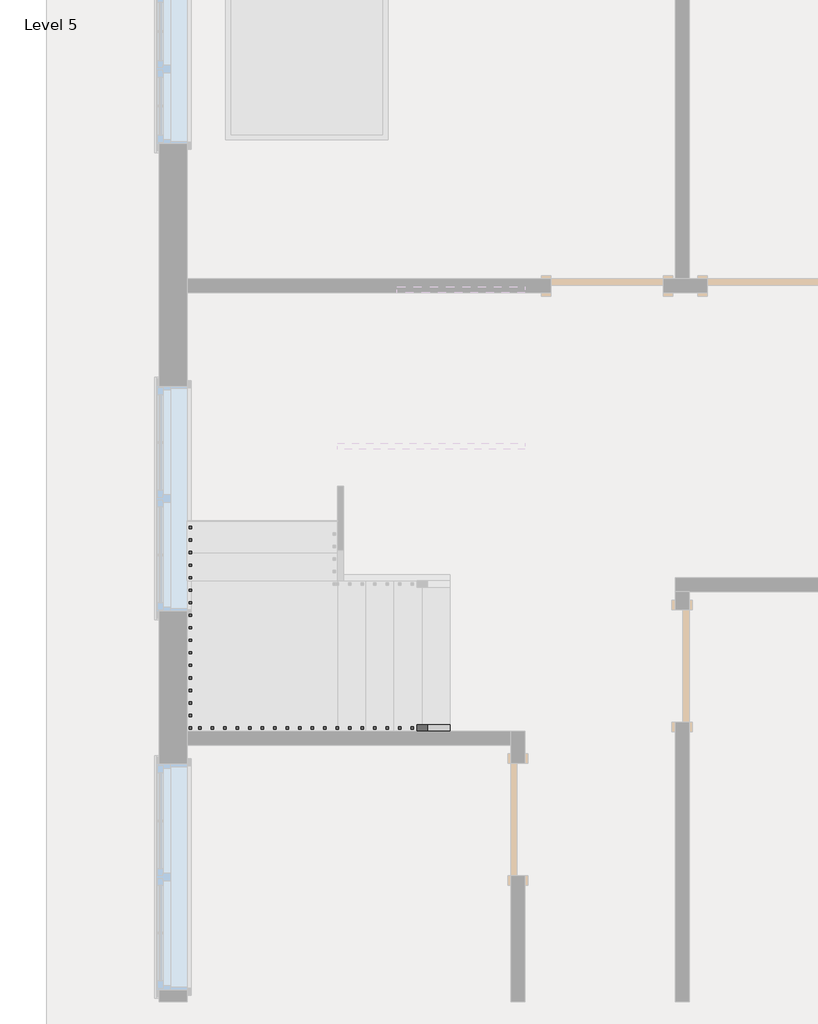
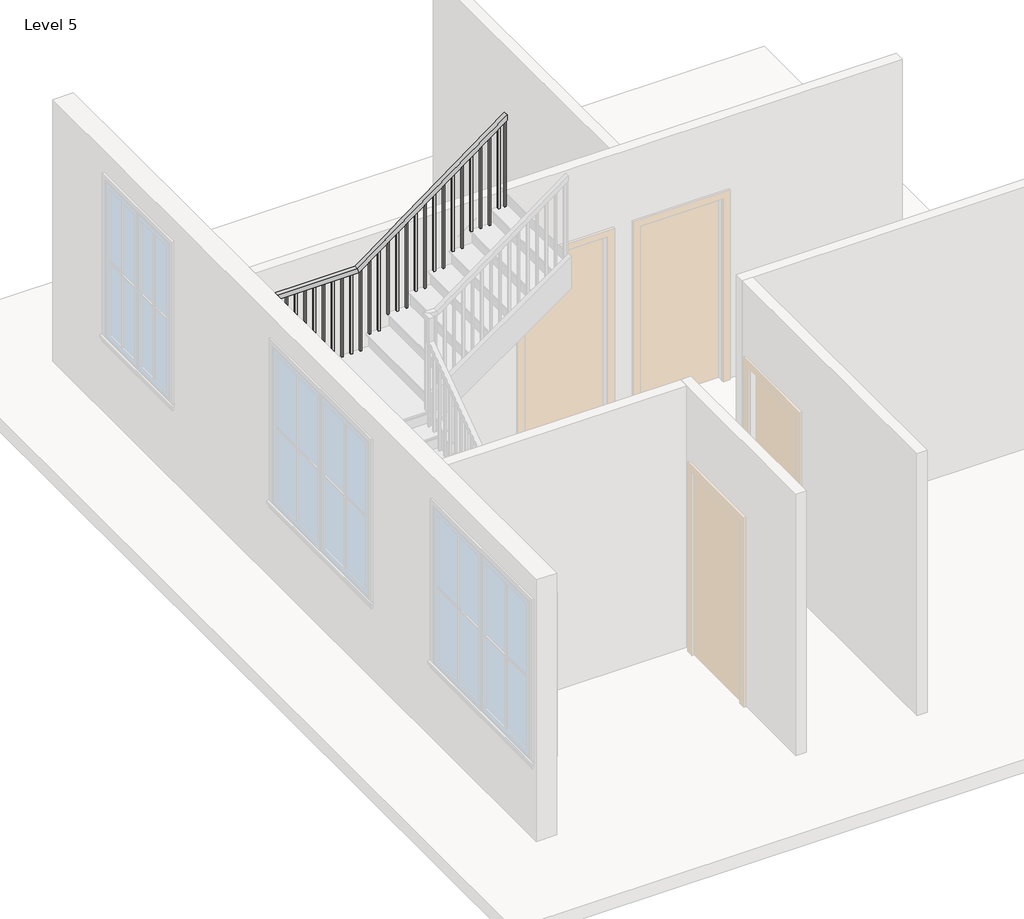
# One storey, part 2 of 3: 1 railing.
"""IFC4 building model written with IfcOpenShell, lengths in millimetres."""

from ifc_helpers import new_model, si_unit, frame, origin, place, context, project, spatial, polyline, outline, extrude, faceted_brep, element, save

model = new_model("IFC4")

# Units and contexts
model_context = context("Model", 3, world=origin())
ifc_project = project(units=[si_unit("LENGTHUNIT", "METRE", prefix="MILLI")], contexts=[model_context])

# Site, building, storey
site = spatial("IfcSite", under=ifc_project)
building = spatial("IfcBuilding", under=site)
storey = spatial("IfcBuildingStorey", under=building, Name="Level 5", Elevation=12649.2)

# Railing
placement = place(None, origin())
element("IfcRailing", 1, ObjectType="Handrail - Rectangular", at=placement, inside=storey, context=model_context, shape_type="SolidModel", body=[
    faceted_brep([(-2683.1105391, -2741.0373761, 13724.0210526), (-2683.1105391, -2741.0373761, 13661.9605986), (-2683.1105391, -2690.2373761, 13661.9605986), (-2683.1105391, -2690.2373761, 13724.0210526), (-3698.24463, -2741.0373761, 14436.3958533), (-3714.290777, -2741.0373761, 14385.5958533), (-3714.290777, -2690.2373761, 14385.5958533), (-3698.24463, -2690.2373761, 14436.3958533), (-4816.7105391, -2741.0373761, 14436.3958533), (-4816.7105391, -2741.0373761, 14385.5958533), (-4765.9105391, -2690.2373761, 14385.5958533), (-4765.9105391, -2690.2373761, 14436.3958533), (-4816.7105391, -1646.8618205, 14436.3958533), (-4816.7105391, -1630.5188912, 14385.5958533), (-4765.9105391, -1630.5188912, 14385.5958533), (-4765.9105391, -1646.8618205, 14436.3958533), (-4816.7105391, -308.3947094, 15397.0181818), (-4816.7105391, -292.0517801, 15346.2181818), (-4765.9105391, -292.0517801, 15346.2181818), (-4765.9105391, -308.3947094, 15397.0181818), (-4816.7105391, 814.9626239, 15397.0181818), (-4816.7105391, 814.9626239, 15346.2181818), (-4765.9105391, 764.1626239, 15346.2181818), (-4765.9105391, 764.1626239, 15397.0181818), (-3721.871578, 814.9626239, 15397.0181818), (-3705.1770744, 814.9626239, 15346.2181818), (-3705.1770744, 764.1626239, 15346.2181818), (-3721.871578, 764.1626239, 15397.0181818), (-2073.5105391, 814.9626239, 16611.6), (-2073.5105391, 764.1626239, 16611.6), (-2073.5105391, 764.1626239, 16548.4987868), (-2073.5105391, 814.9626239, 16548.4987868)], [[[0, 1, 2, 3]], [[1, 0, 4, 5]], [[2, 1, 5, 6]], [[3, 2, 6, 7]], [[0, 3, 7, 4]], [[5, 4, 8, 9]], [[6, 5, 9, 10]], [[7, 6, 10, 11]], [[4, 7, 11, 8]], [[9, 8, 12, 13]], [[10, 9, 13, 14]], [[11, 10, 14, 15]], [[8, 11, 15, 12]], [[13, 12, 16, 17]], [[14, 13, 17, 18]], [[15, 14, 18, 19]], [[12, 15, 19, 16]], [[17, 16, 20, 21]], [[18, 17, 21, 22]], [[19, 18, 22, 23]], [[16, 19, 23, 20]], [[21, 20, 24, 25]], [[22, 21, 25, 26]], [[23, 22, 26, 27]], [[20, 23, 27, 24]], [[28, 29, 30, 31]], [[25, 24, 28, 31]], [[26, 25, 31, 30]], [[27, 26, 30, 29]], [[24, 27, 29, 28]]]),
    extrude(outline(polyline([(16485.3329974, -2159.2355391), (15536.7789474, -2159.2355391), (15536.7789474, -2140.1855391), (16499.3698395, -2140.1855391), (16485.3329974, -2159.2355391)])), frame((0.0, 780.0376239, 0.0), z_axis=(0.0, 1.0, 0.0), x_axis=(0.0, 0.0, 1.0)), (0.0, 0.0, 1.0), 19.05),
    extrude(outline(polyline([(16410.4698395, -2260.8355391), (15376.3578947, -2260.8355391), (15376.3578947, -2241.7855391), (16424.5066816, -2241.7855391), (16410.4698395, -2260.8355391)])), frame((0.0, 780.0376239, 0.0), z_axis=(0.0, 1.0, 0.0), x_axis=(0.0, 0.0, 1.0)), (0.0, 0.0, 1.0), 19.05),
    extrude(outline(polyline([(16335.6066816, -2362.4355391), (15376.3578947, -2362.4355391), (15376.3578947, -2343.3855391), (16349.6435237, -2343.3855391), (16335.6066816, -2362.4355391)])), frame((0.0, 780.0376239, 0.0), z_axis=(0.0, 1.0, 0.0), x_axis=(0.0, 0.0, 1.0)), (0.0, 0.0, 1.0), 19.05),
    extrude(outline(polyline([(16260.7435237, -2464.0355391), (15376.3578947, -2464.0355391), (15376.3578947, -2444.9855391), (16274.7803658, -2444.9855391), (16260.7435237, -2464.0355391)])), frame((0.0, 780.0376239, 0.0), z_axis=(0.0, 1.0, 0.0), x_axis=(0.0, 0.0, 1.0)), (0.0, 0.0, 1.0), 19.05),
    extrude(outline(polyline([(16185.8803658, -2565.6355391), (15215.9368421, -2565.6355391), (15215.9368421, -2546.5855391), (16199.9172079, -2546.5855391), (16185.8803658, -2565.6355391)])), frame((0.0, 780.0376239, 0.0), z_axis=(0.0, 1.0, 0.0), x_axis=(0.0, 0.0, 1.0)), (0.0, 0.0, 1.0), 19.05),
    extrude(outline(polyline([(16111.0172079, -2667.2355391), (15215.9368421, -2667.2355391), (15215.9368421, -2648.1855391), (16125.05405, -2648.1855391), (16111.0172079, -2667.2355391)])), frame((0.0, 780.0376239, 0.0), z_axis=(0.0, 1.0, 0.0), x_axis=(0.0, 0.0, 1.0)), (0.0, 0.0, 1.0), 19.05),
    extrude(outline(polyline([(16036.15405, -2768.8355391), (15055.5157895, -2768.8355391), (15055.5157895, -2749.7855391), (16050.1908921, -2749.7855391), (16036.15405, -2768.8355391)])), frame((0.0, 780.0376239, 0.0), z_axis=(0.0, 1.0, 0.0), x_axis=(0.0, 0.0, 1.0)), (0.0, 0.0, 1.0), 19.05),
    extrude(outline(polyline([(15961.2908921, -2870.4355391), (15055.5157895, -2870.4355391), (15055.5157895, -2851.3855391), (15975.3277342, -2851.3855391), (15961.2908921, -2870.4355391)])), frame((0.0, 780.0376239, 0.0), z_axis=(0.0, 1.0, 0.0), x_axis=(0.0, 0.0, 1.0)), (0.0, 0.0, 1.0), 19.05),
    extrude(outline(polyline([(15886.4277342, -2972.0355391), (14895.0947368, -2972.0355391), (14895.0947368, -2952.9855391), (15900.4645763, -2952.9855391), (15886.4277342, -2972.0355391)])), frame((0.0, 780.0376239, 0.0), z_axis=(0.0, 1.0, 0.0), x_axis=(0.0, 0.0, 1.0)), (0.0, 0.0, 1.0), 19.05),
    extrude(outline(polyline([(15811.5645763, -3073.6355391), (14895.0947368, -3073.6355391), (14895.0947368, -3054.5855391), (15825.6014184, -3054.5855391), (15811.5645763, -3073.6355391)])), frame((0.0, 780.0376239, 0.0), z_axis=(0.0, 1.0, 0.0), x_axis=(0.0, 0.0, 1.0)), (0.0, 0.0, 1.0), 19.05),
    extrude(outline(polyline([(15736.7014184, -3175.2355391), (14734.6736842, -3175.2355391), (14734.6736842, -3156.1855391), (15750.7382605, -3156.1855391), (15736.7014184, -3175.2355391)])), frame((0.0, 780.0376239, 0.0), z_axis=(0.0, 1.0, 0.0), x_axis=(0.0, 0.0, 1.0)), (0.0, 0.0, 1.0), 19.05),
    extrude(outline(polyline([(15661.8382605, -3276.8355391), (14734.6736842, -3276.8355391), (14734.6736842, -3257.7855391), (15675.8751026, -3257.7855391), (15661.8382605, -3276.8355391)])), frame((0.0, 780.0376239, 0.0), z_axis=(0.0, 1.0, 0.0), x_axis=(0.0, 0.0, 1.0)), (0.0, 0.0, 1.0), 19.05),
    extrude(outline(polyline([(15586.9751026, -3378.4355391), (14734.6736842, -3378.4355391), (14734.6736842, -3359.3855391), (15601.0119447, -3359.3855391), (15586.9751026, -3378.4355391)])), frame((0.0, 780.0376239, 0.0), z_axis=(0.0, 1.0, 0.0), x_axis=(0.0, 0.0, 1.0)), (0.0, 0.0, 1.0), 19.05),
    extrude(outline(polyline([(15512.1119447, -3480.0355391), (14574.2526316, -3480.0355391), (14574.2526316, -3460.9855391), (15526.1487868, -3460.9855391), (15512.1119447, -3480.0355391)])), frame((0.0, 780.0376239, 0.0), z_axis=(0.0, 1.0, 0.0), x_axis=(0.0, 0.0, 1.0)), (0.0, 0.0, 1.0), 19.05),
    extrude(outline(polyline([(15437.2487868, -3581.6355391), (14574.2526316, -3581.6355391), (14574.2526316, -3562.5855391), (15451.2856289, -3562.5855391), (15437.2487868, -3581.6355391)])), frame((0.0, 780.0376239, 0.0), z_axis=(0.0, 1.0, 0.0), x_axis=(0.0, 0.0, 1.0)), (0.0, 0.0, 1.0), 19.05),
    extrude(outline(polyline([(15362.3856289, -3683.2355391), (14413.8315789, -3683.2355391), (14413.8315789, -3664.1855391), (15376.422471, -3664.1855391), (15362.3856289, -3683.2355391)])), frame((0.0, 780.0376239, 0.0), z_axis=(0.0, 1.0, 0.0), x_axis=(0.0, 0.0, 1.0)), (0.0, 0.0, 1.0), 19.05),
    extrude(outline(polyline([(-3784.8355391, 799.0876239), (-3765.7855391, 799.0876239), (-3765.7855391, 780.0376239), (-3784.8355391, 780.0376239), (-3784.8355391, 799.0876239)])), frame((0.0, 0.0, 14413.8315789), z_axis=(0.0, 0.0, 1.0), x_axis=(1.0, 0.0, 0.0)), (0.0, 0.0, 1.0), 932.3866029),
    extrude(outline(polyline([(-3886.4355391, 799.0876239), (-3867.3855391, 799.0876239), (-3867.3855391, 780.0376239), (-3886.4355391, 780.0376239), (-3886.4355391, 799.0876239)])), frame((0.0, 0.0, 14413.8315789), z_axis=(0.0, 0.0, 1.0), x_axis=(1.0, 0.0, 0.0)), (0.0, 0.0, 1.0), 932.3866029),
    extrude(outline(polyline([(-3988.0355391, 799.0876239), (-3968.9855391, 799.0876239), (-3968.9855391, 780.0376239), (-3988.0355391, 780.0376239), (-3988.0355391, 799.0876239)])), frame((0.0, 0.0, 14413.8315789), z_axis=(0.0, 0.0, 1.0), x_axis=(1.0, 0.0, 0.0)), (0.0, 0.0, 1.0), 932.3866029),
    extrude(outline(polyline([(-4089.6355391, 799.0876239), (-4070.5855391, 799.0876239), (-4070.5855391, 780.0376239), (-4089.6355391, 780.0376239), (-4089.6355391, 799.0876239)])), frame((0.0, 0.0, 14413.8315789), z_axis=(0.0, 0.0, 1.0), x_axis=(1.0, 0.0, 0.0)), (0.0, 0.0, 1.0), 932.3866029),
    extrude(outline(polyline([(-4191.2355391, 799.0876239), (-4172.1855391, 799.0876239), (-4172.1855391, 780.0376239), (-4191.2355391, 780.0376239), (-4191.2355391, 799.0876239)])), frame((0.0, 0.0, 14413.8315789), z_axis=(0.0, 0.0, 1.0), x_axis=(1.0, 0.0, 0.0)), (0.0, 0.0, 1.0), 932.3866029),
    extrude(outline(polyline([(-4292.8355391, 799.0876239), (-4273.7855391, 799.0876239), (-4273.7855391, 780.0376239), (-4292.8355391, 780.0376239), (-4292.8355391, 799.0876239)])), frame((0.0, 0.0, 14413.8315789), z_axis=(0.0, 0.0, 1.0), x_axis=(1.0, 0.0, 0.0)), (0.0, 0.0, 1.0), 932.3866029),
    extrude(outline(polyline([(-4394.4355391, 799.0876239), (-4375.3855391, 799.0876239), (-4375.3855391, 780.0376239), (-4394.4355391, 780.0376239), (-4394.4355391, 799.0876239)])), frame((0.0, 0.0, 14413.8315789), z_axis=(0.0, 0.0, 1.0), x_axis=(1.0, 0.0, 0.0)), (0.0, 0.0, 1.0), 932.3866029),
    extrude(outline(polyline([(-4496.0355391, 799.0876239), (-4476.9855391, 799.0876239), (-4476.9855391, 780.0376239), (-4496.0355391, 780.0376239), (-4496.0355391, 799.0876239)])), frame((0.0, 0.0, 14413.8315789), z_axis=(0.0, 0.0, 1.0), x_axis=(1.0, 0.0, 0.0)), (0.0, 0.0, 1.0), 932.3866029),
    extrude(outline(polyline([(-4597.6355391, 799.0876239), (-4578.5855391, 799.0876239), (-4578.5855391, 780.0376239), (-4597.6355391, 780.0376239), (-4597.6355391, 799.0876239)])), frame((0.0, 0.0, 14413.8315789), z_axis=(0.0, 0.0, 1.0), x_axis=(1.0, 0.0, 0.0)), (0.0, 0.0, 1.0), 932.3866029),
    extrude(outline(polyline([(-4699.2355391, 799.0876239), (-4680.1855391, 799.0876239), (-4680.1855391, 780.0376239), (-4699.2355391, 780.0376239), (-4699.2355391, 799.0876239)])), frame((0.0, 0.0, 14413.8315789), z_axis=(0.0, 0.0, 1.0), x_axis=(1.0, 0.0, 0.0)), (0.0, 0.0, 1.0), 932.3866029),
    extrude(outline(polyline([(-4800.8355391, 729.2376239), (-4800.8355391, 748.2876239), (-4781.7855391, 748.2876239), (-4781.7855391, 729.2376239), (-4800.8355391, 729.2376239)])), frame((0.0, 0.0, 14413.8315789), z_axis=(0.0, 0.0, 1.0), x_axis=(1.0, 0.0, 0.0)), (0.0, 0.0, 1.0), 932.3866029),
    extrude(outline(polyline([(-4800.8355391, 627.6376239), (-4800.8355391, 646.6876239), (-4781.7855391, 646.6876239), (-4781.7855391, 627.6376239), (-4800.8355391, 627.6376239)])), frame((0.0, 0.0, 14413.8315789), z_axis=(0.0, 0.0, 1.0), x_axis=(1.0, 0.0, 0.0)), (0.0, 0.0, 1.0), 932.3866029),
    extrude(outline(polyline([(-4800.8355391, 526.0376239), (-4800.8355391, 545.0876239), (-4781.7855391, 545.0876239), (-4781.7855391, 526.0376239), (-4800.8355391, 526.0376239)])), frame((0.0, 0.0, 14413.8315789), z_axis=(0.0, 0.0, 1.0), x_axis=(1.0, 0.0, 0.0)), (0.0, 0.0, 1.0), 932.3866029),
    extrude(outline(polyline([(-4800.8355391, 424.4376239), (-4800.8355391, 443.4876239), (-4781.7855391, 443.4876239), (-4781.7855391, 424.4376239), (-4800.8355391, 424.4376239)])), frame((0.0, 0.0, 14413.8315789), z_axis=(0.0, 0.0, 1.0), x_axis=(1.0, 0.0, 0.0)), (0.0, 0.0, 1.0), 932.3866029),
    extrude(outline(polyline([(-4800.8355391, 322.8376239), (-4800.8355391, 341.8876239), (-4781.7855391, 341.8876239), (-4781.7855391, 322.8376239), (-4800.8355391, 322.8376239)])), frame((0.0, 0.0, 14413.8315789), z_axis=(0.0, 0.0, 1.0), x_axis=(1.0, 0.0, 0.0)), (0.0, 0.0, 1.0), 932.3866029),
    extrude(outline(polyline([(-4800.8355391, 221.2376239), (-4800.8355391, 240.2876239), (-4781.7855391, 240.2876239), (-4781.7855391, 221.2376239), (-4800.8355391, 221.2376239)])), frame((0.0, 0.0, 14413.8315789), z_axis=(0.0, 0.0, 1.0), x_axis=(1.0, 0.0, 0.0)), (0.0, 0.0, 1.0), 932.3866029),
    extrude(outline(polyline([(-4800.8355391, 119.6376239), (-4800.8355391, 138.6876239), (-4781.7855391, 138.6876239), (-4781.7855391, 119.6376239), (-4800.8355391, 119.6376239)])), frame((0.0, 0.0, 14413.8315789), z_axis=(0.0, 0.0, 1.0), x_axis=(1.0, 0.0, 0.0)), (0.0, 0.0, 1.0), 932.3866029),
    extrude(outline(polyline([(-4800.8355391, 18.0376239), (-4800.8355391, 37.0876239), (-4781.7855391, 37.0876239), (-4781.7855391, 18.0376239), (-4800.8355391, 18.0376239)])), frame((0.0, 0.0, 14413.8315789), z_axis=(0.0, 0.0, 1.0), x_axis=(1.0, 0.0, 0.0)), (0.0, 0.0, 1.0), 932.3866029),
    extrude(outline(polyline([(-4800.8355391, -83.5623761), (-4800.8355391, -64.5123761), (-4781.7855391, -64.5123761), (-4781.7855391, -83.5623761), (-4800.8355391, -83.5623761)])), frame((0.0, 0.0, 14413.8315789), z_axis=(0.0, 0.0, 1.0), x_axis=(1.0, 0.0, 0.0)), (0.0, 0.0, 1.0), 932.3866029),
    extrude(outline(polyline([(-4800.8355391, -185.1623761), (-4800.8355391, -166.1123761), (-4781.7855391, -166.1123761), (-4781.7855391, -185.1623761), (-4800.8355391, -185.1623761)])), frame((0.0, 0.0, 14413.8315789), z_axis=(0.0, 0.0, 1.0), x_axis=(1.0, 0.0, 0.0)), (0.0, 0.0, 1.0), 932.3866029),
    extrude(outline(polyline([(-4800.8355391, -286.7623761), (-4800.8355391, -267.7123761), (-4781.7855391, -267.7123761), (-4781.7855391, -286.7623761), (-4800.8355391, -286.7623761)])), frame((0.0, 0.0, 14413.8315789), z_axis=(0.0, 0.0, 1.0), x_axis=(1.0, 0.0, 0.0)), (0.0, 0.0, 1.0), 932.3866029),
    extrude(outline(polyline([(-369.3123761, 15290.7679933), (-369.3123761, 14413.8315789), (-388.3623761, 14413.8315789), (-388.3623761, 15277.0957445), (-369.3123761, 15290.7679933)])), frame((-4800.8355391, 0.0, 0.0), z_axis=(1.0, 0.0, 0.0), x_axis=(0.0, 1.0, 0.0)), (0.0, 0.0, 1.0), 19.05),
    extrude(outline(polyline([(-470.9123761, 15217.849333), (-470.9123761, 14253.4105263), (-489.9623761, 14253.4105263), (-489.9623761, 15204.1770842), (-470.9123761, 15217.849333)])), frame((-4800.8355391, 0.0, 0.0), z_axis=(1.0, 0.0, 0.0), x_axis=(0.0, 1.0, 0.0)), (0.0, 0.0, 1.0), 19.05),
    extrude(outline(polyline([(-572.5123761, 15144.9306727), (-572.5123761, 14253.4105263), (-591.5623761, 14253.4105263), (-591.5623761, 15131.2584239), (-572.5123761, 15144.9306727)])), frame((-4800.8355391, 0.0, 0.0), z_axis=(1.0, 0.0, 0.0), x_axis=(0.0, 1.0, 0.0)), (0.0, 0.0, 1.0), 19.05),
    extrude(outline(polyline([(-674.1123761, 15072.0120124), (-674.1123761, 14092.9894737), (-693.1623761, 14092.9894737), (-693.1623761, 15058.3397636), (-674.1123761, 15072.0120124)])), frame((-4800.8355391, 0.0, 0.0), z_axis=(1.0, 0.0, 0.0), x_axis=(0.0, 1.0, 0.0)), (0.0, 0.0, 1.0), 19.05),
    extrude(outline(polyline([(-775.7123761, 14999.0933521), (-775.7123761, 14092.9894737), (-794.7623761, 14092.9894737), (-794.7623761, 14985.4211033), (-775.7123761, 14999.0933521)])), frame((-4800.8355391, 0.0, 0.0), z_axis=(1.0, 0.0, 0.0), x_axis=(0.0, 1.0, 0.0)), (0.0, 0.0, 1.0), 19.05),
    extrude(outline(polyline([(-877.3123761, 14926.1746919), (-877.3123761, 13932.5684211), (-896.3623761, 13932.5684211), (-896.3623761, 14912.502443), (-877.3123761, 14926.1746919)])), frame((-4800.8355391, 0.0, 0.0), z_axis=(1.0, 0.0, 0.0), x_axis=(0.0, 1.0, 0.0)), (0.0, 0.0, 1.0), 19.05),
    extrude(outline(polyline([(-978.9123761, 14853.2560316), (-978.9123761, 13932.5684211), (-997.9623761, 13932.5684211), (-997.9623761, 14839.5837828), (-978.9123761, 14853.2560316)])), frame((-4800.8355391, 0.0, 0.0), z_axis=(1.0, 0.0, 0.0), x_axis=(0.0, 1.0, 0.0)), (0.0, 0.0, 1.0), 19.05),
    extrude(outline(polyline([(-1080.5123761, 14780.3373713), (-1080.5123761, 13772.1473684), (-1099.5623761, 13772.1473684), (-1099.5623761, 14766.6651225), (-1080.5123761, 14780.3373713)])), frame((-4800.8355391, 0.0, 0.0), z_axis=(1.0, 0.0, 0.0), x_axis=(0.0, 1.0, 0.0)), (0.0, 0.0, 1.0), 19.05),
    extrude(outline(polyline([(-1182.1123761, 14707.418711), (-1182.1123761, 13772.1473684), (-1201.1623761, 13772.1473684), (-1201.1623761, 14693.7464622), (-1182.1123761, 14707.418711)])), frame((-4800.8355391, 0.0, 0.0), z_axis=(1.0, 0.0, 0.0), x_axis=(0.0, 1.0, 0.0)), (0.0, 0.0, 1.0), 19.05),
    extrude(outline(polyline([(-1283.7123761, 14634.5000507), (-1283.7123761, 13772.1473684), (-1302.7623761, 13772.1473684), (-1302.7623761, 14620.8278019), (-1283.7123761, 14634.5000507)])), frame((-4800.8355391, 0.0, 0.0), z_axis=(1.0, 0.0, 0.0), x_axis=(0.0, 1.0, 0.0)), (0.0, 0.0, 1.0), 19.05),
    extrude(outline(polyline([(-1385.3123761, 14561.5813904), (-1385.3123761, 13611.7263158), (-1404.3623761, 13611.7263158), (-1404.3623761, 14547.9091416), (-1385.3123761, 14561.5813904)])), frame((-4800.8355391, 0.0, 0.0), z_axis=(1.0, 0.0, 0.0), x_axis=(0.0, 1.0, 0.0)), (0.0, 0.0, 1.0), 19.05),
    extrude(outline(polyline([(-1486.9123761, 14488.6627301), (-1486.9123761, 13611.7263158), (-1505.9623761, 13611.7263158), (-1505.9623761, 14474.9904813), (-1486.9123761, 14488.6627301)])), frame((-4800.8355391, 0.0, 0.0), z_axis=(1.0, 0.0, 0.0), x_axis=(0.0, 1.0, 0.0)), (0.0, 0.0, 1.0), 19.05),
    extrude(outline(polyline([(-1588.5123761, 14415.7440698), (-1588.5123761, 13451.3052632), (-1607.5623761, 13451.3052632), (-1607.5623761, 14402.071821), (-1588.5123761, 14415.7440698)])), frame((-4800.8355391, 0.0, 0.0), z_axis=(1.0, 0.0, 0.0), x_axis=(0.0, 1.0, 0.0)), (0.0, 0.0, 1.0), 19.05),
    extrude(outline(polyline([(-4800.8355391, -1709.1623761), (-4800.8355391, -1690.1123761), (-4781.7855391, -1690.1123761), (-4781.7855391, -1709.1623761), (-4800.8355391, -1709.1623761)])), frame((0.0, 0.0, 13451.3052632), z_axis=(0.0, 0.0, 1.0), x_axis=(1.0, 0.0, 0.0)), (0.0, 0.0, 1.0), 934.2905901),
    extrude(outline(polyline([(-4800.8355391, -1810.7623761), (-4800.8355391, -1791.7123761), (-4781.7855391, -1791.7123761), (-4781.7855391, -1810.7623761), (-4800.8355391, -1810.7623761)])), frame((0.0, 0.0, 13451.3052632), z_axis=(0.0, 0.0, 1.0), x_axis=(1.0, 0.0, 0.0)), (0.0, 0.0, 1.0), 934.2905901),
    extrude(outline(polyline([(-4800.8355391, -1912.3623761), (-4800.8355391, -1893.3123761), (-4781.7855391, -1893.3123761), (-4781.7855391, -1912.3623761), (-4800.8355391, -1912.3623761)])), frame((0.0, 0.0, 13451.3052632), z_axis=(0.0, 0.0, 1.0), x_axis=(1.0, 0.0, 0.0)), (0.0, 0.0, 1.0), 934.2905901),
    extrude(outline(polyline([(-4800.8355391, -2013.9623761), (-4800.8355391, -1994.9123761), (-4781.7855391, -1994.9123761), (-4781.7855391, -2013.9623761), (-4800.8355391, -2013.9623761)])), frame((0.0, 0.0, 13451.3052632), z_axis=(0.0, 0.0, 1.0), x_axis=(1.0, 0.0, 0.0)), (0.0, 0.0, 1.0), 934.2905901),
    extrude(outline(polyline([(-4800.8355391, -2115.5623761), (-4800.8355391, -2096.5123761), (-4781.7855391, -2096.5123761), (-4781.7855391, -2115.5623761), (-4800.8355391, -2115.5623761)])), frame((0.0, 0.0, 13451.3052632), z_axis=(0.0, 0.0, 1.0), x_axis=(1.0, 0.0, 0.0)), (0.0, 0.0, 1.0), 934.2905901),
    extrude(outline(polyline([(-4800.8355391, -2217.1623761), (-4800.8355391, -2198.1123761), (-4781.7855391, -2198.1123761), (-4781.7855391, -2217.1623761), (-4800.8355391, -2217.1623761)])), frame((0.0, 0.0, 13451.3052632), z_axis=(0.0, 0.0, 1.0), x_axis=(1.0, 0.0, 0.0)), (0.0, 0.0, 1.0), 934.2905901),
    extrude(outline(polyline([(-4800.8355391, -2318.7623761), (-4800.8355391, -2299.7123761), (-4781.7855391, -2299.7123761), (-4781.7855391, -2318.7623761), (-4800.8355391, -2318.7623761)])), frame((0.0, 0.0, 13451.3052632), z_axis=(0.0, 0.0, 1.0), x_axis=(1.0, 0.0, 0.0)), (0.0, 0.0, 1.0), 934.2905901),
    extrude(outline(polyline([(-4800.8355391, -2420.3623761), (-4800.8355391, -2401.3123761), (-4781.7855391, -2401.3123761), (-4781.7855391, -2420.3623761), (-4800.8355391, -2420.3623761)])), frame((0.0, 0.0, 13451.3052632), z_axis=(0.0, 0.0, 1.0), x_axis=(1.0, 0.0, 0.0)), (0.0, 0.0, 1.0), 934.2905901),
    extrude(outline(polyline([(-4800.8355391, -2521.9623761), (-4800.8355391, -2502.9123761), (-4781.7855391, -2502.9123761), (-4781.7855391, -2521.9623761), (-4800.8355391, -2521.9623761)])), frame((0.0, 0.0, 13451.3052632), z_axis=(0.0, 0.0, 1.0), x_axis=(1.0, 0.0, 0.0)), (0.0, 0.0, 1.0), 934.2905901),
    extrude(outline(polyline([(-4800.8355391, -2623.5623761), (-4800.8355391, -2604.5123761), (-4781.7855391, -2604.5123761), (-4781.7855391, -2623.5623761), (-4800.8355391, -2623.5623761)])), frame((0.0, 0.0, 13451.3052632), z_axis=(0.0, 0.0, 1.0), x_axis=(1.0, 0.0, 0.0)), (0.0, 0.0, 1.0), 934.2905901),
    extrude(outline(polyline([(-4705.5855391, -2725.1623761), (-4724.6355391, -2725.1623761), (-4724.6355391, -2706.1123761), (-4705.5855391, -2706.1123761), (-4705.5855391, -2725.1623761)])), frame((0.0, 0.0, 13451.3052632), z_axis=(0.0, 0.0, 1.0), x_axis=(1.0, 0.0, 0.0)), (0.0, 0.0, 1.0), 934.2905901),
    extrude(outline(polyline([(-4603.9855391, -2725.1623761), (-4623.0355391, -2725.1623761), (-4623.0355391, -2706.1123761), (-4603.9855391, -2706.1123761), (-4603.9855391, -2725.1623761)])), frame((0.0, 0.0, 13451.3052632), z_axis=(0.0, 0.0, 1.0), x_axis=(1.0, 0.0, 0.0)), (0.0, 0.0, 1.0), 934.2905901),
    extrude(outline(polyline([(-4502.3855391, -2725.1623761), (-4521.4355391, -2725.1623761), (-4521.4355391, -2706.1123761), (-4502.3855391, -2706.1123761), (-4502.3855391, -2725.1623761)])), frame((0.0, 0.0, 13451.3052632), z_axis=(0.0, 0.0, 1.0), x_axis=(1.0, 0.0, 0.0)), (0.0, 0.0, 1.0), 934.2905901),
    extrude(outline(polyline([(-4400.7855391, -2725.1623761), (-4419.8355391, -2725.1623761), (-4419.8355391, -2706.1123761), (-4400.7855391, -2706.1123761), (-4400.7855391, -2725.1623761)])), frame((0.0, 0.0, 13451.3052632), z_axis=(0.0, 0.0, 1.0), x_axis=(1.0, 0.0, 0.0)), (0.0, 0.0, 1.0), 934.2905901),
    extrude(outline(polyline([(-4299.1855391, -2725.1623761), (-4318.2355391, -2725.1623761), (-4318.2355391, -2706.1123761), (-4299.1855391, -2706.1123761), (-4299.1855391, -2725.1623761)])), frame((0.0, 0.0, 13451.3052632), z_axis=(0.0, 0.0, 1.0), x_axis=(1.0, 0.0, 0.0)), (0.0, 0.0, 1.0), 934.2905901),
    extrude(outline(polyline([(-4197.5855391, -2725.1623761), (-4216.6355391, -2725.1623761), (-4216.6355391, -2706.1123761), (-4197.5855391, -2706.1123761), (-4197.5855391, -2725.1623761)])), frame((0.0, 0.0, 13451.3052632), z_axis=(0.0, 0.0, 1.0), x_axis=(1.0, 0.0, 0.0)), (0.0, 0.0, 1.0), 934.2905901),
    extrude(outline(polyline([(-4095.9855391, -2725.1623761), (-4115.0355391, -2725.1623761), (-4115.0355391, -2706.1123761), (-4095.9855391, -2706.1123761), (-4095.9855391, -2725.1623761)])), frame((0.0, 0.0, 13451.3052632), z_axis=(0.0, 0.0, 1.0), x_axis=(1.0, 0.0, 0.0)), (0.0, 0.0, 1.0), 934.2905901),
    extrude(outline(polyline([(-3994.3855391, -2725.1623761), (-4013.4355391, -2725.1623761), (-4013.4355391, -2706.1123761), (-3994.3855391, -2706.1123761), (-3994.3855391, -2725.1623761)])), frame((0.0, 0.0, 13451.3052632), z_axis=(0.0, 0.0, 1.0), x_axis=(1.0, 0.0, 0.0)), (0.0, 0.0, 1.0), 934.2905901),
    extrude(outline(polyline([(-3892.7855391, -2725.1623761), (-3911.8355391, -2725.1623761), (-3911.8355391, -2706.1123761), (-3892.7855391, -2706.1123761), (-3892.7855391, -2725.1623761)])), frame((0.0, 0.0, 13451.3052632), z_axis=(0.0, 0.0, 1.0), x_axis=(1.0, 0.0, 0.0)), (0.0, 0.0, 1.0), 934.2905901),
    extrude(outline(polyline([(-3791.1855391, -2725.1623761), (-3810.2355391, -2725.1623761), (-3810.2355391, -2706.1123761), (-3791.1855391, -2706.1123761), (-3791.1855391, -2725.1623761)])), frame((0.0, 0.0, 13451.3052632), z_axis=(0.0, 0.0, 1.0), x_axis=(1.0, 0.0, 0.0)), (0.0, 0.0, 1.0), 934.2905901),
    extrude(outline(polyline([(-3689.5855391, -2725.1623761), (-3708.6355391, -2725.1623761), (-3708.6355391, -2706.1123761), (-3689.5855391, -2706.1123761), (-3689.5855391, -2725.1623761)])), frame((0.0, 0.0, 13451.3052632), z_axis=(0.0, 0.0, 1.0), x_axis=(1.0, 0.0, 0.0)), (0.0, 0.0, 1.0), 934.2905901),
    extrude(outline(polyline([(14310.3290196, -3607.0355391), (13451.3052632, -3607.0355391), (13451.3052632, -3587.9855391), (14296.9605986, -3587.9855391), (14310.3290196, -3607.0355391)])), frame((0.0, -2725.1623761, 0.0), z_axis=(0.0, 1.0, 0.0), x_axis=(0.0, 0.0, 1.0)), (0.0, 0.0, 1.0), 19.05),
    extrude(outline(polyline([(14239.030774, -3505.4355391), (13290.8842105, -3505.4355391), (13290.8842105, -3486.3855391), (14225.662353, -3486.3855391), (14239.030774, -3505.4355391)])), frame((0.0, -2725.1623761, 0.0), z_axis=(0.0, 1.0, 0.0), x_axis=(0.0, 0.0, 1.0)), (0.0, 0.0, 1.0), 19.05),
    extrude(outline(polyline([(14167.7325284, -3403.8355391), (13290.8842105, -3403.8355391), (13290.8842105, -3384.7855391), (14154.3641074, -3384.7855391), (14167.7325284, -3403.8355391)])), frame((0.0, -2725.1623761, 0.0), z_axis=(0.0, 1.0, 0.0), x_axis=(0.0, 0.0, 1.0)), (0.0, 0.0, 1.0), 19.05),
    extrude(outline(polyline([(14096.4342828, -3302.2355391), (13130.4631579, -3302.2355391), (13130.4631579, -3283.1855391), (14083.0658617, -3283.1855391), (14096.4342828, -3302.2355391)])), frame((0.0, -2725.1623761, 0.0), z_axis=(0.0, 1.0, 0.0), x_axis=(0.0, 0.0, 1.0)), (0.0, 0.0, 1.0), 19.05),
    extrude(outline(polyline([(14025.1360372, -3200.6355391), (13130.4631579, -3200.6355391), (13130.4631579, -3181.5855391), (14011.7676161, -3181.5855391), (14025.1360372, -3200.6355391)])), frame((0.0, -2725.1623761, 0.0), z_axis=(0.0, 1.0, 0.0), x_axis=(0.0, 0.0, 1.0)), (0.0, 0.0, 1.0), 19.05),
    extrude(outline(polyline([(13953.8377916, -3099.0355391), (12970.0421053, -3099.0355391), (12970.0421053, -3079.9855391), (13940.4693705, -3079.9855391), (13953.8377916, -3099.0355391)])), frame((0.0, -2725.1623761, 0.0), z_axis=(0.0, 1.0, 0.0), x_axis=(0.0, 0.0, 1.0)), (0.0, 0.0, 1.0), 19.05),
    extrude(outline(polyline([(13882.5395459, -2997.4355391), (12970.0421053, -2997.4355391), (12970.0421053, -2978.3855391), (13869.1711249, -2978.3855391), (13882.5395459, -2997.4355391)])), frame((0.0, -2725.1623761, 0.0), z_axis=(0.0, 1.0, 0.0), x_axis=(0.0, 0.0, 1.0)), (0.0, 0.0, 1.0), 19.05),
    extrude(outline(polyline([(13811.2413003, -2895.8355391), (12809.6210526, -2895.8355391), (12809.6210526, -2876.7855391), (13797.8728793, -2876.7855391), (13811.2413003, -2895.8355391)])), frame((0.0, -2725.1623761, 0.0), z_axis=(0.0, 1.0, 0.0), x_axis=(0.0, 0.0, 1.0)), (0.0, 0.0, 1.0), 19.05),
    extrude(outline(polyline([(13739.9430547, -2794.2355391), (12809.6210526, -2794.2355391), (12809.6210526, -2775.1855391), (13726.5746337, -2775.1855391), (13739.9430547, -2794.2355391)])), frame((0.0, -2725.1623761, 0.0), z_axis=(0.0, 1.0, 0.0), x_axis=(0.0, 0.0, 1.0)), (0.0, 0.0, 1.0), 19.05),
    extrude(outline(polyline([(-4800.8355391, 780.0376239), (-4800.8355391, 799.0876239), (-4781.7855391, 799.0876239), (-4781.7855391, 780.0376239), (-4800.8355391, 780.0376239)])), frame((0.0, 0.0, 14413.8315789), z_axis=(0.0, 0.0, 1.0), x_axis=(1.0, 0.0, 0.0)), (0.0, 0.0, 1.0), 932.3866029),
    extrude(outline(polyline([(-4781.7855391, -2725.1623761), (-4800.8355391, -2725.1623761), (-4800.8355391, -2706.1123761), (-4781.7855391, -2706.1123761), (-4781.7855391, -2725.1623761)])), frame((0.0, 0.0, 13451.3052632), z_axis=(0.0, 0.0, 1.0), x_axis=(1.0, 0.0, 0.0)), (0.0, 0.0, 1.0), 934.2905901),
    extrude(outline(polyline([(16534.4619447, -2092.5605391), (15536.7789474, -2092.5605391), (15536.7789474, -2073.5105391), (16548.4987868, -2073.5105391), (16534.4619447, -2092.5605391)])), frame((0.0, 780.0376239, 0.0), z_axis=(0.0, 1.0, 0.0), x_axis=(0.0, 0.0, 1.0)), (0.0, 0.0, 1.0), 19.05),
    extrude(outline(polyline([(13675.3290196, -2702.1605391), (12809.6210526, -2702.1605391), (12809.6210526, -2683.1105391), (13661.9605986, -2683.1105391), (13675.3290196, -2702.1605391)])), frame((0.0, -2725.1623761, 0.0), z_axis=(0.0, 1.0, 0.0), x_axis=(0.0, 0.0, 1.0)), (0.0, 0.0, 1.0), 19.05),
])

save(model, "model.ifc")

# Revit data of these elements
# Type "Handrail - Rectangular"
#   Assembly Code = "C2010400"
#   built-in parameter 1008612 = 0.0416667 (stored number, unit not read)
#   built-in parameter 1008611 = 0.0416667 (stored number, unit not read)
#   built-in parameter 1008609 = 0.333333 (stored number, unit not read)
#   built-in parameter 1008604 = 0.166667 (stored number, unit not read)
#   built-in parameter 1008603 = 0.166667 (stored number, unit not read)
#   Railing Height = 3' - 0"
#   built-in parameter 1008630 = 2
#   built-in parameter 1008610 = 2
#   built-in parameter 1008618 = Baluster - Square : 3/4"
# Element 1 (IfcRailing, "Handrail - Rectangular")
#   Phase Created = New Construction
